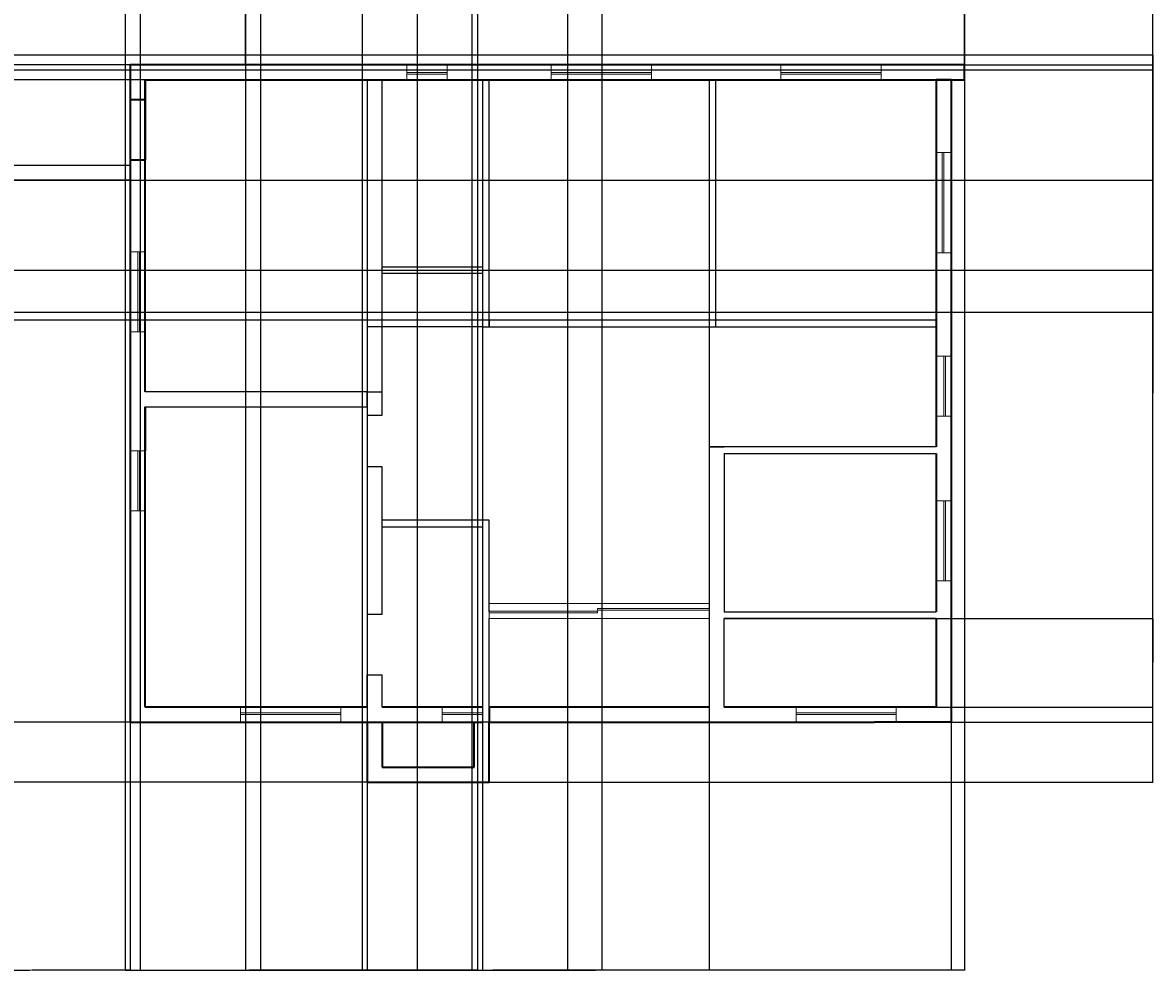
# Model space of a CAD drawing. Units: inches. Extents: x 2029 to 8798, y 1998 to 6373.
# Tile 6 of 11: x 3826 to 4504, y 4031 to 4599. Entities that reach past the tile are written whole.
import ezdxf

# ---------------------------------------------------------------- set-up
doc = ezdxf.new("R2010")
doc.units = ezdxf.units.IN
for name, color, linetype, lineweight in [('A-ANNO-DIMS', 2, 'Continuous', 18), ('A-GLAZ', 4, 'Continuous', 18), ('A-WALL-CIRC', 7, 'Continuous', 25), ('A-WALL-EXTR', 7, 'Continuous', 35), ('A-WALL-INTR', 7, 'Continuous', 25)]:
    doc.layers.add(name, color=color, linetype=linetype, lineweight=lineweight)
doc.styles.get("Standard").update_dxf_attribs({"font": 'arial.ttf'})
doc.dimstyles.get("Standard").update_dxf_attribs({"dimtxt": 0.18, "dimasz": 0.18, "dimexe": 0.18, "dimexo": 0.0625, "dimgap": 0.09, "dimtad": 0, "dimtih": 1, "dimtoh": 1, "dimdec": 4, "dimzin": 0, "dimdsep": 46, "dimtxsty": 'Standard', "dimcen": 0.09, "dimadec": 0, "dimazin": 0, "dimtfac": 1, "dimtdec": 4, "dimtofl": 0, "dimtmove": 0, "dimatfit": 3, "dimfxl": 1, "dimtolj": 1, "dimtzin": 0, "dimarcsym": 0})

# ---------------------------------------------------------------- blocks, each defined once
blk = doc.blocks.new('WIN-60')
for p, q in [((0, 0), (0, 9)), ((60, 9), (60, 0)), ((0, 4.5), (60, 4.5)), ((0, 3.5), (60, 3.5))]:
    blk.add_line(p, q)
blk = doc.blocks.new('WIN-36')
for p, q in [((0, 36), (9, 36)), ((3.5, 36), (3.5, 0)), ((4.5, 36), (4.5, 0)), ((9, 0), (0, 0))]:
    blk.add_line(p, q)
blk = doc.blocks.new('WIN-48')
for p, q in [((0, 48), (9, 48)), ((4.5, 48), (4.5, 0)), ((5.5, 48), (5.5, 0)), ((9, 0), (0, 0))]:
    blk.add_line(p, q)
blk = doc.blocks.new('WIN-24')
for p, q in [((0, 0), (0, 9)), ((24, 9), (24, 0)), ((0, 4.5), (24, 4.5)), ((0, 3.5), (24, 3.5))]:
    blk.add_line(p, q)
blk = doc.blocks.new('*D41')
at = {"layer": 'A-ANNO-DIMS', "color": 0, "lineweight": -2, "transparency": 16777216}
for p, q in [((3771.77, 4209.93), (3771.77, 4031.06)), ((3890.77, 4179.93), (3890.77, 4031.06)), ((3771.95, 4031.24), (3830.99, 4031.24)), ((3890.59, 4031.24), (3831.55, 4031.24))]:
    blk.add_line(p, q, dxfattribs=at)
at = {"layer": 'A-ANNO-DIMS', "color": 0, "transparency": 16777216}
for points in [[(3771.95, 4031.27), (3771.95, 4031.21), (3771.77, 4031.24)], [(3890.59, 4031.27), (3890.59, 4031.21), (3890.77, 4031.24)]]:
    blk.add_solid(points, dxfattribs=at)
at = {"layer": 'Defpoints', "color": 0, "transparency": 16777216}
for p in [(3771.77, 4209.99), (3890.77, 4179.99), (3890.77, 4031.24)]:
    blk.add_point(p, dxfattribs=at)
at = {"layer": 'A-ANNO-DIMS', "color": 0, "transparency": 16777216, "insert": (3831.27, 4031.24), "char_height": 0.18, "attachment_point": 5}
blk.add_mtext('\\A1;119', dxfattribs=at)
blk = doc.blocks.new('*D42')
at = {"layer": 'A-ANNO-DIMS', "color": 0, "lineweight": -2, "transparency": 16777216}
for p, q in [((3890.77, 4179.93), (3890.77, 4031.06)), ((4382.77, 4179.93), (4382.77, 4031.06)), ((3890.95, 4031.24), (4136.47, 4031.24)), ((4382.59, 4031.24), (4137.06, 4031.24))]:
    blk.add_line(p, q, dxfattribs=at)
at = {"layer": 'A-ANNO-DIMS', "color": 0, "transparency": 16777216}
for points in [[(3890.95, 4031.27), (3890.95, 4031.21), (3890.77, 4031.24)], [(4382.59, 4031.27), (4382.59, 4031.21), (4382.77, 4031.24)]]:
    blk.add_solid(points, dxfattribs=at)
at = {"layer": 'Defpoints', "color": 0, "transparency": 16777216}
for p in [(3890.77, 4179.99), (4382.77, 4179.99), (4382.77, 4031.24)]:
    blk.add_point(p, dxfattribs=at)
at = {"layer": 'A-ANNO-DIMS', "color": 0, "transparency": 16777216, "insert": (4136.77, 4031.24), "char_height": 0.18, "attachment_point": 5}
blk.add_mtext('\\A1;492', dxfattribs=at)
blk = doc.blocks.new('*D52')
at = {"layer": 'A-ANNO-DIMS', "color": 0, "lineweight": -2, "transparency": 16777216}
for p, q in [((2861.6, 4570.99), (4503.7, 4570.99)), ((4503.52, 4570.81), (4503.52, 4511.17)), ((4503.52, 4451.17), (4503.52, 4510.81)), ((2861.6, 4450.99), (4503.7, 4450.99))]:
    blk.add_line(p, q, dxfattribs=at)
at = {"layer": 'A-ANNO-DIMS', "color": 0, "transparency": 16777216}
for points in [[(4503.49, 4570.81), (4503.55, 4570.81), (4503.52, 4570.99)], [(4503.49, 4451.17), (4503.55, 4451.17), (4503.52, 4450.99)]]:
    blk.add_solid(points, dxfattribs=at)
at = {"layer": 'Defpoints', "color": 0, "transparency": 16777216}
for p in [(2861.54, 4570.99), (4503.52, 4570.99), (2861.54, 4450.99)]:
    blk.add_point(p, dxfattribs=at)
at = {"layer": 'A-ANNO-DIMS', "color": 0, "transparency": 16777216, "insert": (4503.52, 4510.99), "char_height": 0.18, "attachment_point": 5}
blk.add_mtext('\\A1;120', dxfattribs=at)
blk = doc.blocks.new('*D57')
at = {"layer": 'A-ANNO-DIMS', "color": 0, "lineweight": -2, "transparency": 16777216}
for p, q in [((3771.83, 4579.99), (4503.7, 4579.99)), ((4503.52, 4579.81), (4503.52, 4542.67)), ((4503.52, 4505.17), (4503.52, 4542.31)), ((3771.83, 4504.99), (4503.7, 4504.99))]:
    blk.add_line(p, q, dxfattribs=at)
at = {"layer": 'A-ANNO-DIMS', "color": 0, "transparency": 16777216}
for points in [[(4503.49, 4579.81), (4503.55, 4579.81), (4503.52, 4579.99)], [(4503.49, 4505.17), (4503.55, 4505.17), (4503.52, 4504.99)]]:
    blk.add_solid(points, dxfattribs=at)
at = {"layer": 'Defpoints', "color": 0, "transparency": 16777216}
for p in [(3771.77, 4579.99), (3771.77, 4504.99), (4503.52, 4504.99)]:
    blk.add_point(p, dxfattribs=at)
at = {"layer": 'A-ANNO-DIMS', "color": 0, "transparency": 16777216, "insert": (4503.52, 4542.49), "char_height": 0.18, "attachment_point": 5}
blk.add_mtext('\\A1;75', dxfattribs=at)
blk = doc.blocks.new('*D58')
at = {"layer": 'A-ANNO-DIMS', "color": 0, "lineweight": -2, "transparency": 16777216}
for p, q in [((3771.83, 4450.99), (4503.7, 4450.99)), ((4503.52, 4450.81), (4503.52, 4438.52)), ((4503.52, 4425.88), (4503.52, 4438.16)), ((3771.83, 4425.7), (4503.7, 4425.7))]:
    blk.add_line(p, q, dxfattribs=at)
at = {"layer": 'A-ANNO-DIMS', "color": 0, "transparency": 16777216}
for points in [[(4503.49, 4450.81), (4503.55, 4450.81), (4503.52, 4450.99)], [(4503.49, 4425.88), (4503.55, 4425.88), (4503.52, 4425.7)]]:
    blk.add_solid(points, dxfattribs=at)
at = {"layer": 'Defpoints', "color": 0, "transparency": 16777216}
for p in [(3771.77, 4450.99), (3771.77, 4425.7), (4503.52, 4425.7)]:
    blk.add_point(p, dxfattribs=at)
at = {"layer": 'A-ANNO-DIMS', "color": 0, "transparency": 16777216, "insert": (4503.52, 4438.34), "char_height": 0.18, "attachment_point": 5}
blk.add_mtext('\\A1;25.293', dxfattribs=at)
blk = doc.blocks.new('*D71')
at = {"layer": 'A-ANNO-DIMS', "color": 0, "lineweight": -2, "transparency": 16777216}
for p, q in [((4173.45, 4679.09), (4503.7, 4679.09)), ((4503.52, 4678.91), (4503.52, 4626.72)), ((4503.52, 4574.17), (4503.52, 4626.36)), ((4390.83, 4573.99), (4503.7, 4573.99))]:
    blk.add_line(p, q, dxfattribs=at)
at = {"layer": 'A-ANNO-DIMS', "color": 0, "transparency": 16777216}
for points in [[(4503.49, 4678.91), (4503.55, 4678.91), (4503.52, 4679.09)], [(4503.49, 4574.17), (4503.55, 4574.17), (4503.52, 4573.99)]]:
    blk.add_solid(points, dxfattribs=at)
at = {"layer": 'Defpoints', "color": 0, "transparency": 16777216}
for p in [(4173.39, 4679.09), (4503.52, 4679.09), (4390.77, 4573.99)]:
    blk.add_point(p, dxfattribs=at)
at = {"layer": 'A-ANNO-DIMS', "color": 0, "transparency": 16777216, "insert": (4503.52, 4626.54), "char_height": 0.18, "attachment_point": 5}
blk.add_mtext('\\A1;105.1', dxfattribs=at)
blk = doc.blocks.new('*D76')
at = {"layer": 'A-ANNO-DIMS', "color": 0, "lineweight": -2, "transparency": 16777216}
for p, q in [((3887.77, 5813.55), (3887.77, 4031.06)), ((4390.77, 5813.55), (4390.77, 4031.06)), ((3887.95, 4031.24), (4138.98, 4031.24)), ((4390.59, 4031.24), (4139.55, 4031.24))]:
    blk.add_line(p, q, dxfattribs=at)
at = {"layer": 'A-ANNO-DIMS', "color": 0, "transparency": 16777216}
for points in [[(3887.95, 4031.27), (3887.95, 4031.21), (3887.77, 4031.24)], [(4390.59, 4031.27), (4390.59, 4031.21), (4390.77, 4031.24)]]:
    blk.add_solid(points, dxfattribs=at)
at = {"layer": 'Defpoints', "color": 0, "transparency": 16777216}
for p in [(3887.77, 5813.61), (4390.77, 5813.61), (4390.77, 4031.24)]:
    blk.add_point(p, dxfattribs=at)
at = {"layer": 'A-ANNO-DIMS', "color": 0, "transparency": 16777216, "insert": (4139.27, 4031.24), "char_height": 0.18, "attachment_point": 5}
blk.add_mtext('\\A1;503', dxfattribs=at)
blk = doc.blocks.new('*D78')
at = {"layer": 'A-ANNO-DIMS', "color": 0, "lineweight": -2, "transparency": 16777216}
for p, q in [((3896.77, 6211.55), (3896.77, 4031.06)), ((4029.77, 6211.55), (4029.77, 4031.06)), ((3896.95, 4031.24), (3962.99, 4031.24)), ((4029.59, 4031.24), (3963.55, 4031.24))]:
    blk.add_line(p, q, dxfattribs=at)
at = {"layer": 'A-ANNO-DIMS', "color": 0, "transparency": 16777216}
for points in [[(3896.95, 4031.27), (3896.95, 4031.21), (3896.77, 4031.24)], [(4029.59, 4031.27), (4029.59, 4031.21), (4029.77, 4031.24)]]:
    blk.add_solid(points, dxfattribs=at)
at = {"layer": 'Defpoints', "color": 0, "transparency": 16777216}
for p in [(3896.77, 6211.61), (4029.77, 6211.61), (4029.77, 4031.24)]:
    blk.add_point(p, dxfattribs=at)
at = {"layer": 'A-ANNO-DIMS', "color": 0, "transparency": 16777216, "insert": (3963.27, 4031.24), "char_height": 0.18, "attachment_point": 5}
blk.add_mtext('\\A1;133', dxfattribs=at)
blk = doc.blocks.new('*D83')
at = {"layer": 'A-ANNO-DIMS', "color": 0, "lineweight": -2, "transparency": 16777216}
for p, q in [((4062.77, 6151.55), (4062.77, 4031.06)), ((4152.77, 6151.55), (4152.77, 4031.06)), ((4062.95, 4031.24), (4107.55, 4031.24)), ((4152.59, 4031.24), (4107.98, 4031.24))]:
    blk.add_line(p, q, dxfattribs=at)
at = {"layer": 'A-ANNO-DIMS', "color": 0, "transparency": 16777216}
for points in [[(4062.95, 4031.27), (4062.95, 4031.21), (4062.77, 4031.24)], [(4152.59, 4031.27), (4152.59, 4031.21), (4152.77, 4031.24)]]:
    blk.add_solid(points, dxfattribs=at)
at = {"layer": 'Defpoints', "color": 0, "transparency": 16777216}
for p in [(4062.77, 6151.61), (4152.77, 6151.61), (4152.77, 4031.24)]:
    blk.add_point(p, dxfattribs=at)
at = {"layer": 'A-ANNO-DIMS', "color": 0, "transparency": 16777216, "insert": (4107.77, 4031.24), "char_height": 0.18, "attachment_point": 5}
blk.add_mtext('\\A1;90', dxfattribs=at)
blk = doc.blocks.new('*D84')
at = {"layer": 'A-ANNO-DIMS', "color": 0, "lineweight": -2, "transparency": 16777216}
for p, q in [((3890.77, 4573.93), (3890.77, 4031.06)), ((4032.77, 4564.93), (4032.77, 4031.06)), ((3890.95, 4031.24), (3961.49, 4031.24)), ((4032.59, 4031.24), (3962.05, 4031.24))]:
    blk.add_line(p, q, dxfattribs=at)
at = {"layer": 'A-ANNO-DIMS', "color": 0, "transparency": 16777216}
for points in [[(3890.95, 4031.27), (3890.95, 4031.21), (3890.77, 4031.24)], [(4032.59, 4031.27), (4032.59, 4031.21), (4032.77, 4031.24)]]:
    blk.add_solid(points, dxfattribs=at)
at = {"layer": 'Defpoints', "color": 0, "transparency": 16777216}
for p in [(3890.77, 4573.99), (4032.77, 4564.99), (4032.77, 4031.24)]:
    blk.add_point(p, dxfattribs=at)
at = {"layer": 'A-ANNO-DIMS', "color": 0, "transparency": 16777216, "insert": (3961.77, 4031.24), "char_height": 0.18, "attachment_point": 5}
blk.add_mtext('\\A1;142', dxfattribs=at)
blk = doc.blocks.new('*D85')
at = {"layer": 'A-ANNO-DIMS', "color": 0, "lineweight": -2, "transparency": 16777216}
for p, q in [((4101.77, 4564.93), (4101.77, 4031.06)), ((4237.77, 4564.93), (4237.77, 4031.06)), ((4101.95, 4031.24), (4169.49, 4031.24)), ((4237.59, 4031.24), (4170.05, 4031.24))]:
    blk.add_line(p, q, dxfattribs=at)
at = {"layer": 'A-ANNO-DIMS', "color": 0, "transparency": 16777216}
for points in [[(4101.95, 4031.27), (4101.95, 4031.21), (4101.77, 4031.24)], [(4237.59, 4031.27), (4237.59, 4031.21), (4237.77, 4031.24)]]:
    blk.add_solid(points, dxfattribs=at)
at = {"layer": 'Defpoints', "color": 0, "transparency": 16777216}
for p in [(4101.77, 4564.99), (4237.77, 4564.99), (4237.77, 4031.24)]:
    blk.add_point(p, dxfattribs=at)
at = {"layer": 'A-ANNO-DIMS', "color": 0, "transparency": 16777216, "insert": (4169.77, 4031.24), "char_height": 0.18, "attachment_point": 5}
blk.add_mtext('\\A1;136', dxfattribs=at)
blk = doc.blocks.new('*D86')
at = {"layer": 'A-ANNO-DIMS', "color": 0, "lineweight": -2, "transparency": 16777216}
for p, q in [((4373.7, 4564.99), (2029.61, 4564.99)), ((2029.79, 4564.81), (2029.79, 4493.17)), ((2029.79, 4421.17), (2029.79, 4492.81)), ((4373.7, 4420.99), (2029.61, 4420.99))]:
    blk.add_line(p, q, dxfattribs=at)
at = {"layer": 'A-ANNO-DIMS', "color": 0, "transparency": 16777216}
for points in [[(2029.76, 4564.81), (2029.82, 4564.81), (2029.79, 4564.99)], [(2029.76, 4421.17), (2029.82, 4421.17), (2029.79, 4420.99)]]:
    blk.add_solid(points, dxfattribs=at)
at = {"layer": 'Defpoints', "color": 0, "transparency": 16777216}
for p in [(4373.77, 4564.99), (2029.79, 4420.99), (4373.77, 4420.99)]:
    blk.add_point(p, dxfattribs=at)
at = {"layer": 'A-ANNO-DIMS', "color": 0, "transparency": 16777216, "insert": (2029.79, 4492.99), "char_height": 0.18, "attachment_point": 5}
blk.add_mtext('\\A1;144', dxfattribs=at)
blk = doc.blocks.new('*D87')
at = {"layer": 'A-ANNO-DIMS', "color": 0, "lineweight": -2, "transparency": 16777216}
for p, q in [((4390.83, 4573.99), (4503.7, 4573.99)), ((4503.52, 4573.81), (4503.52, 4377.17)), ((4503.52, 4180.17), (4503.52, 4376.81)), ((4382.83, 4179.99), (4503.7, 4179.99))]:
    blk.add_line(p, q, dxfattribs=at)
at = {"layer": 'A-ANNO-DIMS', "color": 0, "transparency": 16777216}
for points in [[(4503.49, 4573.81), (4503.55, 4573.81), (4503.52, 4573.99)], [(4503.49, 4180.17), (4503.55, 4180.17), (4503.52, 4179.99)]]:
    blk.add_solid(points, dxfattribs=at)
at = {"layer": 'Defpoints', "color": 0, "transparency": 16777216}
for p in [(4390.77, 4573.99), (4503.52, 4573.99), (4382.77, 4179.99)]:
    blk.add_point(p, dxfattribs=at)
at = {"layer": 'A-ANNO-DIMS', "color": 0, "transparency": 16777216, "insert": (4503.52, 4376.99), "char_height": 0.18, "attachment_point": 5}
blk.add_mtext('\\A1;394', dxfattribs=at)
blk = doc.blocks.new('*D88')
at = {"layer": 'A-ANNO-DIMS', "color": 0, "lineweight": -2, "transparency": 16777216}
for p, q in [((2142.54, 4445.05), (2142.54, 6372.54)), ((2142.72, 6372.36), (3266.19, 6372.36)), ((4390.59, 6372.36), (3267.12, 6372.36)), ((4390.77, 4574.05), (4390.77, 6372.54))]:
    blk.add_line(p, q, dxfattribs=at)
at = {"layer": 'A-ANNO-DIMS', "color": 0, "transparency": 16777216}
for points in [[(2142.72, 6372.39), (2142.72, 6372.33), (2142.54, 6372.36)], [(4390.59, 6372.39), (4390.59, 6372.33), (4390.77, 6372.36)]]:
    blk.add_solid(points, dxfattribs=at)
at = {"layer": 'Defpoints', "color": 0, "transparency": 16777216}
for p in [(4390.77, 6372.36), (4390.77, 4573.99), (2142.54, 4444.99)]:
    blk.add_point(p, dxfattribs=at)
at = {"layer": 'A-ANNO-DIMS', "color": 0, "transparency": 16777216, "insert": (3266.65, 6372.36), "char_height": 0.18, "attachment_point": 5}
blk.add_mtext('\\A1;2248.2', dxfattribs=at)
blk = doc.blocks.new('*D89')
at = {"layer": 'A-ANNO-DIMS', "color": 0, "lineweight": -2, "transparency": 16777216}
for p, q in [((4249.83, 6259.61), (4503.7, 6259.61)), ((4503.52, 6259.43), (4503.52, 5201.98)), ((4503.52, 4144.17), (4503.52, 5201.62)), ((4105.83, 4143.99), (4503.7, 4143.99))]:
    blk.add_line(p, q, dxfattribs=at)
at = {"layer": 'A-ANNO-DIMS', "color": 0, "transparency": 16777216}
for points in [[(4503.49, 6259.43), (4503.55, 6259.43), (4503.52, 6259.61)], [(4503.49, 4144.17), (4503.55, 4144.17), (4503.52, 4143.99)]]:
    blk.add_solid(points, dxfattribs=at)
at = {"layer": 'Defpoints', "color": 0, "transparency": 16777216}
for p in [(4249.77, 6259.61), (4503.52, 6259.61), (4105.77, 4143.99)]:
    blk.add_point(p, dxfattribs=at)
at = {"layer": 'A-ANNO-DIMS', "color": 0, "transparency": 16777216, "insert": (4503.52, 5201.8), "char_height": 0.18, "attachment_point": 5}
blk.add_mtext('\\A1;2115.6', dxfattribs=at)
blk = doc.blocks.new('*D90')
at = {"layer": 'A-ANNO-DIMS', "color": 0, "lineweight": -2, "transparency": 16777216}
for p, q in [((4095.39, 4679.03), (4095.39, 4031.06)), ((4173.39, 4679.03), (4173.39, 4031.06)), ((4095.57, 4031.24), (4134.17, 4031.24)), ((4173.21, 4031.24), (4134.61, 4031.24))]:
    blk.add_line(p, q, dxfattribs=at)
at = {"layer": 'A-ANNO-DIMS', "color": 0, "transparency": 16777216}
for points in [[(4095.57, 4031.27), (4095.57, 4031.21), (4095.39, 4031.24)], [(4173.21, 4031.27), (4173.21, 4031.21), (4173.39, 4031.24)]]:
    blk.add_solid(points, dxfattribs=at)
at = {"layer": 'Defpoints', "color": 0, "transparency": 16777216}
for p in [(4095.39, 4679.09), (4173.39, 4679.09), (4173.39, 4031.24)]:
    blk.add_point(p, dxfattribs=at)
at = {"layer": 'A-ANNO-DIMS', "color": 0, "transparency": 16777216, "insert": (4134.39, 4031.24), "char_height": 0.18, "attachment_point": 5}
blk.add_mtext('\\A1;78', dxfattribs=at)
blk = doc.blocks.new('*D92')
at = {"layer": 'A-ANNO-DIMS', "color": 0, "lineweight": -2, "transparency": 16777216}
for p, q in [((3959.77, 4736.03), (3959.77, 4031.06)), ((4095.39, 4679.03), (4095.39, 4031.06)), ((3959.95, 4031.24), (4027.12, 4031.24)), ((4095.21, 4031.24), (4028.03, 4031.24))]:
    blk.add_line(p, q, dxfattribs=at)
at = {"layer": 'A-ANNO-DIMS', "color": 0, "transparency": 16777216}
for points in [[(3959.95, 4031.27), (3959.95, 4031.21), (3959.77, 4031.24)], [(4095.21, 4031.27), (4095.21, 4031.21), (4095.39, 4031.24)]]:
    blk.add_solid(points, dxfattribs=at)
at = {"layer": 'Defpoints', "color": 0, "transparency": 16777216}
for p in [(3959.77, 4736.09), (4095.39, 4679.09), (4095.39, 4031.24)]:
    blk.add_point(p, dxfattribs=at)
at = {"layer": 'A-ANNO-DIMS', "color": 0, "transparency": 16777216, "insert": (4027.58, 4031.24), "char_height": 0.18, "attachment_point": 5}
blk.add_mtext('\\A1;135.62', dxfattribs=at)
blk = doc.blocks.new('*D107')
at = {"layer": 'A-ANNO-DIMS', "color": 0, "lineweight": -2, "transparency": 16777216}
for p, q in [((3968.77, 5479.55), (3968.77, 4031.06)), ((4098.77, 5479.55), (4098.77, 4031.06)), ((3968.95, 4031.24), (4033.49, 4031.24)), ((4098.59, 4031.24), (4034.05, 4031.24))]:
    blk.add_line(p, q, dxfattribs=at)
at = {"layer": 'A-ANNO-DIMS', "color": 0, "transparency": 16777216}
for points in [[(3968.95, 4031.27), (3968.95, 4031.21), (3968.77, 4031.24)], [(4098.59, 4031.27), (4098.59, 4031.21), (4098.77, 4031.24)]]:
    blk.add_solid(points, dxfattribs=at)
at = {"layer": 'Defpoints', "color": 0, "transparency": 16777216}
for p in [(3968.77, 5479.61), (4098.77, 5479.61), (4098.77, 4031.24)]:
    blk.add_point(p, dxfattribs=at)
at = {"layer": 'A-ANNO-DIMS', "color": 0, "transparency": 16777216, "insert": (4033.77, 4031.24), "char_height": 0.18, "attachment_point": 5}
blk.add_mtext('\\A1;130', dxfattribs=at)
blk = doc.blocks.new('*D116')
at = {"layer": 'A-ANNO-DIMS', "color": 0, "lineweight": -2, "transparency": 16777216}
for p, q in [((4246.83, 4241.99), (4503.7, 4241.99)), ((4503.52, 4241.81), (4503.52, 4215.67)), ((4503.52, 4189.17), (4503.52, 4215.31)), ((4246.83, 4188.99), (4503.7, 4188.99))]:
    blk.add_line(p, q, dxfattribs=at)
at = {"layer": 'A-ANNO-DIMS', "color": 0, "transparency": 16777216}
for points in [[(4503.49, 4241.81), (4503.55, 4241.81), (4503.52, 4241.99)], [(4503.49, 4189.17), (4503.55, 4189.17), (4503.52, 4188.99)]]:
    blk.add_solid(points, dxfattribs=at)
at = {"layer": 'Defpoints', "color": 0, "transparency": 16777216}
for p in [(4246.77, 4241.99), (4503.52, 4241.99), (4246.77, 4188.99)]:
    blk.add_point(p, dxfattribs=at)
at = {"layer": 'A-ANNO-DIMS', "color": 0, "transparency": 16777216, "insert": (4503.52, 4215.49), "char_height": 0.18, "attachment_point": 5}
blk.add_mtext('\\A1;53', dxfattribs=at)
blk = doc.blocks.new('*D117')
at = {"layer": 'A-ANNO-DIMS', "color": 0, "lineweight": -2, "transparency": 16777216}
for p, q in [((4105.7, 4179.99), (2029.61, 4179.99)), ((2029.79, 4179.81), (2029.79, 4162.17)), ((2029.79, 4144.17), (2029.79, 4161.81)), ((4105.7, 4143.99), (2029.61, 4143.99))]:
    blk.add_line(p, q, dxfattribs=at)
at = {"layer": 'A-ANNO-DIMS', "color": 0, "transparency": 16777216}
for points in [[(2029.76, 4179.81), (2029.82, 4179.81), (2029.79, 4179.99)], [(2029.76, 4144.17), (2029.82, 4144.17), (2029.79, 4143.99)]]:
    blk.add_solid(points, dxfattribs=at)
at = {"layer": 'Defpoints', "color": 0, "transparency": 16777216}
for p in [(2029.79, 4179.99), (4105.77, 4179.99), (4105.77, 4143.99)]:
    blk.add_point(p, dxfattribs=at)
at = {"layer": 'A-ANNO-DIMS', "color": 0, "transparency": 16777216, "insert": (2029.79, 4161.99), "char_height": 0.18, "attachment_point": 5}
blk.add_mtext('\\A1;36', dxfattribs=at)

msp = doc.modelspace()

# ---------------------------------------------------------------- linework, layer by layer
at = {"layer": 'A-GLAZ'}
for p, q in [((4056.5828, 4573.9886), (4080.5828, 4573.9886)), ((4143.0841, 4573.9886), (4203.0841, 4573.9886)), ((4280.6777, 4573.9886), (4340.6777, 4573.9886)), ((4373.7657, 4521.4248), (4373.7657, 4461.4248)), ((3890.7657, 4413.9886), (3890.7657, 4461.9886)), ((4382.7657, 4399.3479), (4382.7657, 4363.3479)), ((3890.7657, 4342.613), (3890.7657, 4306.613)), ((4382.7657, 4312.7224), (4382.7657, 4264.7224)), ((4105.7657, 4241.9886), (4105.7657, 4250.9886)), ((4105.7657, 4250.9886), (4237.7657, 4250.9886)), ((4237.7657, 4250.9886), (4237.7657, 4241.9886)), ((4105.7657, 4246.4886), (4170.7657, 4246.4886)), ((4170.7657, 4245.4886), (4105.7657, 4245.4886)), ((4237.7657, 4247.9886), (4170.7657, 4247.9886)), ((4170.7657, 4247.9886), (4170.7657, 4246.9886)), ((4170.7657, 4246.9886), (4237.7657, 4246.9886)), ((4170.7657, 4246.4886), (4170.7657, 4245.4886)), ((4237.7657, 4246.9886), (4237.7657, 4247.9886)), ((4237.7657, 4241.9886), (4105.7657, 4241.9886)), ((4101.7657, 4188.9886), (4077.7657, 4188.9886)), ((4016.8933, 4179.9886), (3956.8933, 4179.9886)), ((4349.7657, 4179.9886), (4289.7657, 4179.9886))]:
    msp.add_line(p, q, dxfattribs=at)
at = {"layer": 'A-WALL-CIRC'}
for p, q in [((3968.7657, 4736.0948), (3968.7657, 4573.9886)), ((3959.7657, 4573.9886), (3959.7657, 4616.0948)), ((3890.7657, 4573.9886), (3771.7657, 4573.9886)), ((3762.7657, 4513.9886), (3890.7657, 4513.9886)), ((3890.7657, 4504.9886), (3770.7657, 4504.9886))]:
    msp.add_line(p, q, dxfattribs=at)
at = {"layer": 'A-WALL-EXTR'}
for p, q in [((3899.7657, 4573.9886), (3890.7657, 4573.9886)), ((3890.7657, 4573.9886), (3890.7657, 4564.9886)), ((3959.7657, 4573.9886), (3899.7657, 4573.9886)), ((3968.7657, 4573.9886), (3959.7657, 4573.9886)), ((4390.7657, 4573.9886), (3968.7657, 4573.9886)), ((4390.7657, 4564.9886), (4390.7657, 4573.9886)), ((3890.7657, 4564.9886), (3890.7657, 4363.9886)), ((3899.7657, 4564.9886), (3968.7657, 4564.9886)), ((3899.7657, 4564.9886), (4032.7657, 4564.9886)), ((3899.7657, 4377.9886), (3899.7657, 4564.9886)), ((3899.7657, 4564.9886), (3899.7657, 4540.9886)), ((3899.7657, 4564.9886), (3899.7657, 4552.9886)), ((3968.7657, 4564.9886), (4040.7657, 4564.9886)), ((4040.7657, 4564.9886), (4049.7657, 4564.9886)), ((4041.7657, 4564.9886), (4101.7657, 4564.9886)), ((4041.7657, 4564.9886), (4056.5828, 4564.9886)), ((4049.7657, 4564.9886), (4109.7657, 4564.9886)), ((4105.7657, 4564.9886), (4237.7657, 4564.9886)), ((4105.7657, 4564.9886), (4143.0841, 4564.9886)), ((4109.7657, 4564.9886), (4113.7657, 4564.9886)), ((4113.7657, 4564.9886), (4245.7657, 4564.9886)), ((4241.7657, 4564.9886), (4373.7657, 4564.9886)), ((4241.7657, 4564.9886), (4280.6777, 4564.9886)), ((4245.7657, 4564.9886), (4249.7657, 4564.9886)), ((4249.7657, 4564.9886), (4381.7657, 4564.9886)), ((4373.7657, 4564.9886), (4382.7657, 4564.9886)), ((4382.7657, 4564.9886), (4373.7657, 4564.9886)), ((4373.7657, 4564.9886), (4373.7657, 4344.9886)), ((4373.7657, 4564.9886), (4373.7657, 4420.9886)), ((4381.7657, 4564.9886), (4390.7657, 4564.9886)), ((4382.7657, 4564.9886), (4382.7657, 4179.9886)), ((4382.7657, 4564.9886), (4382.7657, 4521.4248)), ((3899.7657, 4552.9886), (3890.7657, 4552.9886)), ((3899.7657, 4552.9886), (3899.7657, 4516.9886)), ((3899.7657, 4516.9886), (3890.7657, 4516.9886)), ((3890.7657, 4516.9886), (3890.7657, 4504.9886)), ((3899.7657, 4377.9886), (3899.7657, 4413.9886)), ((4373.7657, 4416.9886), (4373.7657, 4344.9886)), ((4373.7657, 4416.9886), (4373.7657, 4399.3479)), ((3890.7657, 4363.9886), (3890.7657, 4359.9886)), ((3899.7657, 4188.9886), (3899.7657, 4368.9886)), ((3899.7657, 4188.9886), (3899.7657, 4368.9886)), ((3899.7657, 4368.9886), (3899.7657, 4342.613)), ((3890.7657, 4359.9886), (3890.7657, 4179.9886)), ((4373.7657, 4340.9886), (4373.7657, 4245.9886)), ((4373.7657, 4340.9886), (4373.7657, 4312.7224)), ((4373.7657, 4241.9886), (4373.7657, 4188.9886)), ((4032.7657, 4188.9886), (3899.7657, 4188.9886)), ((3899.7657, 4188.9886), (3899.7657, 4188.9886)), ((4032.7657, 4188.9886), (4016.8933, 4188.9886)), ((4101.7657, 4188.9886), (4041.7657, 4188.9886)), ((4101.7657, 4188.9886), (4041.7657, 4188.9886)), ((4237.7657, 4188.9886), (4105.7657, 4188.9886)), ((4105.7657, 4188.9886), (4105.7657, 4179.9886)), ((4373.7657, 4188.9886), (4246.7657, 4188.9886)), ((4373.7657, 4188.9886), (4349.7657, 4188.9886)), ((3890.7657, 4179.9886), (3899.7657, 4179.9886)), ((3899.7657, 4179.9886), (3908.7657, 4179.9886)), ((3908.7657, 4179.9886), (4041.7657, 4179.9886)), ((4032.7657, 4179.9886), (4032.7657, 4143.9886)), ((4041.7657, 4179.9886), (4050.7657, 4179.9886)), ((4041.7657, 4179.9886), (4041.7657, 4152.9886)), ((4050.7657, 4179.9886), (4054.7657, 4179.9886)), ((4054.7657, 4179.9886), (4101.7657, 4179.9886)), ((4096.7657, 4152.9886), (4096.7657, 4179.9886)), ((4105.7657, 4143.9886), (4105.7657, 4179.9886)), ((4105.7657, 4179.9886), (4186.7657, 4179.9886)), ((4186.7657, 4179.9886), (4195.7657, 4179.9886)), ((4195.7657, 4179.9886), (4327.7657, 4179.9886)), ((4327.7657, 4179.9886), (4336.7657, 4179.9886)), ((4382.7657, 4179.9886), (4336.7657, 4179.9886)), ((4041.7657, 4152.9886), (4096.7657, 4152.9886)), ((4032.7657, 4143.9886), (4105.7657, 4143.9886))]:
    msp.add_line(p, q, dxfattribs=at)
at = {"layer": 'A-WALL-INTR'}
for p, q in [((4032.7657, 4564.9886), (4032.7657, 4416.9886)), ((4041.7657, 4363.9886), (4041.7657, 4564.9886)), ((4101.7657, 4564.9886), (4101.7657, 4416.9886)), ((4105.7657, 4416.9886), (4105.7657, 4564.9886)), ((4237.7657, 4564.9886), (4237.7657, 4420.9886)), ((4241.7657, 4416.9886), (4241.7657, 4564.9886)), ((4041.7657, 4416.9886), (4041.7657, 4452.9886)), ((4041.7657, 4452.9886), (4101.7657, 4452.9886)), ((4101.7657, 4452.9886), (4101.7657, 4448.9886)), ((4101.7657, 4448.9886), (4041.7657, 4448.9886)), ((4237.7657, 4420.9886), (4105.7657, 4420.9886)), ((4105.7657, 4420.9886), (4105.7657, 4416.9886)), ((4373.7657, 4420.9886), (4237.7657, 4420.9886)), ((4237.7657, 4420.9886), (4237.7657, 4416.9886)), ((4101.7657, 4416.9886), (4032.7657, 4416.9886)), ((4101.7657, 4416.9886), (4105.7657, 4416.9886)), ((4105.7657, 4416.9886), (4237.7657, 4416.9886)), ((4237.7657, 4416.9886), (4241.7657, 4416.9886)), ((4237.7657, 4416.9886), (4373.7657, 4416.9886)), ((4032.7657, 4377.9886), (3899.7657, 4377.9886)), ((4032.7657, 4368.9886), (4032.7657, 4377.9886)), ((4032.7657, 4377.9886), (4032.7657, 4363.9886)), ((4032.7657, 4377.9886), (4041.7657, 4377.9886)), ((3899.7657, 4368.9886), (4032.7657, 4368.9886)), ((4032.7657, 4363.9886), (4041.7657, 4363.9886)), ((4241.7657, 4344.9886), (4237.7657, 4344.9886)), ((4237.7657, 4344.9886), (4237.7657, 4245.9886)), ((4237.7657, 4344.9886), (4246.7657, 4344.9886)), ((4237.7657, 4344.9886), (4237.7657, 4340.9886)), ((4373.7657, 4344.9886), (4241.7657, 4344.9886)), ((4246.7657, 4340.9886), (4246.7657, 4245.9886)), ((4246.7657, 4340.9886), (4373.7657, 4340.9886)), ((4041.7657, 4332.9886), (4032.7657, 4332.9886)), ((4032.7657, 4332.9886), (4032.7657, 4188.9886)), ((4041.7657, 4296.9886), (4041.7657, 4332.9886)), ((4101.7657, 4300.9886), (4041.7657, 4300.9886)), ((4041.7657, 4296.9886), (4101.7657, 4296.9886)), ((4041.7657, 4244.3791), (4041.7657, 4296.9886)), ((4105.7657, 4300.9886), (4101.7657, 4300.9886)), ((4101.7657, 4296.9886), (4101.7657, 4245.9886)), ((4105.7657, 4296.9886), (4105.7657, 4300.9886)), ((4105.7657, 4245.9886), (4105.7657, 4296.9886)), ((4041.7657, 4244.3791), (4032.7657, 4244.3791)), ((4101.7657, 4245.9886), (4101.7657, 4188.9886)), ((4246.7657, 4245.9886), (4373.7657, 4245.9886)), ((4105.7657, 4188.9886), (4105.7657, 4241.9886)), ((4105.7657, 4188.9886), (4105.7657, 4241.9886)), ((4237.7657, 4241.9886), (4237.7657, 4188.9886)), ((4373.7657, 4241.9886), (4246.7657, 4241.9886)), ((4246.7657, 4188.9886), (4246.7657, 4241.9886)), ((4032.7657, 4188.9886), (4032.7657, 4208.3791)), ((4032.7657, 4208.3791), (4041.7657, 4208.3791)), ((4041.7657, 4188.9886), (4041.7657, 4208.3791))]:
    msp.add_line(p, q, dxfattribs=at)

# ---------------------------------------------------------------- block references
at = {"layer": 'A-GLAZ'}
for name, p in [('WIN-24', (4056.5828, 4564.9886)), ('WIN-60', (4143.0841, 4564.9886)), ('WIN-60', (4280.6777, 4564.9886)), ('WIN-48', (3890.7657, 4413.9886)), ('WIN-48', (4373.7657, 4264.7224))]:
    msp.add_blockref(name, p, dxfattribs=at)
at = {"layer": 'A-GLAZ', "extrusion": (0, 0, -1), "zscale": -1}
for name, p, rotation in [('WIN-60', (-4373.7657, 4461.4248), 90), ('WIN-60', (-3956.8933, 4188.9886), 180), ('WIN-24', (-4077.7657, 4188.9886), 180), ('WIN-60', (-4289.7657, 4188.9886), 180)]:
    msp.add_blockref(name, p, dxfattribs=dict(at, rotation=rotation))
for p in [(-4382.7657, 4363.3479), (-3899.7657, 4306.613)]:
    msp.add_blockref('WIN-36', p, dxfattribs=at)

# ---------------------------------------------------------------- dimensions: what is measured, and where the dimension line sits
at = {"layer": 'A-ANNO-DIMS'}
for base, p1, p2, override, picture, middle in [((4390.7657, 6372.3623), (2142.5398, 4444.9886), (4390.7657, 4573.9886), {"dimdec": 1, "dimlfac": 1, "dimrnd": 0, "dimzin": 0, "dimdsep": 46, "dimlunit": 2}, '*D88', (3266.6528, 6372.3623)), ((4029.7657, 4031.2386), (3896.7657, 6211.6123), (4029.7657, 6211.6123), {"dimdec": 0, "dimlfac": 1, "dimrnd": 0, "dimzin": 0, "dimdsep": 46, "dimlunit": 2}, '*D78', (3963.2657, 4031.2386)), ((4152.7657, 4031.2386), (4062.7657, 6151.6123), (4152.7657, 6151.6123), {"dimdec": 0, "dimlfac": 1, "dimrnd": 0, "dimzin": 0, "dimdsep": 46, "dimlunit": 2}, '*D83', (4107.7657, 4031.2386)), ((4390.7657, 4031.2386), (3887.7657, 5813.6123), (4390.7657, 5813.6123), {"dimdec": 0, "dimlfac": 1, "dimrnd": 0, "dimzin": 0, "dimdsep": 46, "dimlunit": 2}, '*D76', (4139.2657, 4031.2386)), ((4098.7657, 4031.2386), (3968.7657, 5479.6123), (4098.7657, 5479.6123), {"dimdec": 0, "dimlfac": 1, "dimrnd": 0, "dimzin": 0, "dimdsep": 46, "dimlunit": 2}, '*D107', (4033.7657, 4031.2386)), ((4095.3869, 4031.2386), (3959.7657, 4736.0948), (4095.3869, 4679.0948), {"dimdec": 2, "dimlfac": 1, "dimrnd": 0, "dimzin": 0, "dimdsep": 46, "dimlunit": 2}, '*D92', (4027.5763, 4031.2386)), ((4173.3869, 4031.2386), (4095.3869, 4679.0948), (4173.3869, 4679.0948), {"dimdec": 0, "dimlfac": 1, "dimrnd": 0, "dimzin": 0, "dimdsep": 46, "dimlunit": 2}, '*D90', (4134.3869, 4031.2386)), ((4032.7657, 4031.2386), (3890.7657, 4573.9886), (4032.7657, 4564.9886), {"dimdec": 0, "dimlfac": 1, "dimrnd": 0, "dimzin": 0, "dimdsep": 46, "dimlunit": 2}, '*D84', (3961.7657, 4031.2386)), ((4237.7657, 4031.2386), (4101.7657, 4564.9886), (4237.7657, 4564.9886), {"dimdec": 0, "dimlfac": 1, "dimrnd": 0, "dimzin": 0, "dimdsep": 46, "dimlunit": 2}, '*D85', (4169.7657, 4031.2386)), ((3890.7657, 4031.2386), (3771.7657, 4209.9886), (3890.7657, 4179.9886), {"dimdec": 0, "dimlfac": 1, "dimrnd": 0, "dimzin": 0, "dimdsep": 46, "dimlunit": 2}, '*D41', (3831.2657, 4031.2386)), ((4382.7657, 4031.2386), (3890.7657, 4179.9886), (4382.7657, 4179.9886), {"dimdec": 0, "dimlfac": 1, "dimrnd": 0, "dimzin": 0, "dimdsep": 46, "dimlunit": 2}, '*D42', (4136.7657, 4031.2386))]:
    dim = msp.add_linear_dim(base=base, p1=p1, p2=p2, dimstyle='Standard', override=override, dxfattribs=at)
    dim.commit()
    dim.dimension.update_dxf_attribs({"geometry": picture, "text_midpoint": middle})
for base, p1, p2, override, picture, middle in [((4503.5157, 6259.6123), (4105.7657, 4143.9886), (4249.7657, 6259.6123), {"dimdec": 1, "dimlfac": 1, "dimrnd": 0, "dimzin": 0, "dimdsep": 46, "dimlunit": 2}, '*D89', (4503.5157, 5201.8004)), ((4503.5157, 4679.0948), (4390.7657, 4573.9886), (4173.3869, 4679.0948), {"dimdec": 1, "dimlfac": 1, "dimrnd": 0, "dimzin": 0, "dimdsep": 46, "dimlunit": 2}, '*D71', (4503.5157, 4626.5417)), ((4503.5157, 4504.9886), (3771.7657, 4579.9886), (3771.7657, 4504.9886), {"dimdec": 0, "dimlfac": 1, "dimrnd": 0, "dimzin": 0, "dimdsep": 46, "dimlunit": 2}, '*D57', (4503.5157, 4542.4886)), ((4503.5157, 4570.9886), (2861.5398, 4450.9886), (2861.5398, 4570.9886), {"dimdec": 0, "dimlfac": 1, "dimrnd": 0, "dimzin": 0, "dimdsep": 46, "dimlunit": 2}, '*D52', (4503.5157, 4510.9886)), ((4503.5157, 4573.9886), (4382.7657, 4179.9886), (4390.7657, 4573.9886), {"dimdec": 0, "dimlfac": 1, "dimrnd": 0, "dimzin": 0, "dimdsep": 46, "dimlunit": 2}, '*D87', (4503.5157, 4376.9886)), ((2029.7898, 4420.9886), (4373.7657, 4564.9886), (4373.7657, 4420.9886), {"dimdec": 0, "dimlfac": 1, "dimrnd": 0, "dimzin": 0, "dimdsep": 46, "dimlunit": 2}, '*D86', (2029.7898, 4492.9886)), ((4503.5157, 4425.6956), (3771.7657, 4450.9886), (3771.7657, 4425.6956), {"dimdec": 3, "dimlfac": 1, "dimrnd": 0, "dimzin": 0, "dimdsep": 46, "dimlunit": 2}, '*D58', (4503.5157, 4438.3421)), ((4503.5157, 4241.9886), (4246.7657, 4188.9886), (4246.7657, 4241.9886), {"dimdec": 0, "dimlfac": 1, "dimrnd": 0, "dimzin": 0, "dimdsep": 46, "dimlunit": 2}, '*D116', (4503.5157, 4215.4886)), ((2029.7898, 4179.9886), (4105.7657, 4143.9886), (4105.7657, 4179.9886), {"dimdec": 0, "dimlfac": 1, "dimrnd": 0, "dimzin": 0, "dimdsep": 46, "dimlunit": 2}, '*D117', (2029.7898, 4161.9886))]:
    dim = msp.add_linear_dim(base=base, p1=p1, p2=p2, angle=90, dimstyle='Standard', override=override, dxfattribs=at)
    dim.commit()
    dim.dimension.update_dxf_attribs({"geometry": picture, "text_midpoint": middle})

doc.saveas('drawing.dxf')
